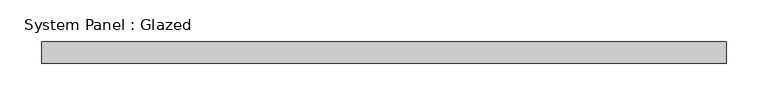
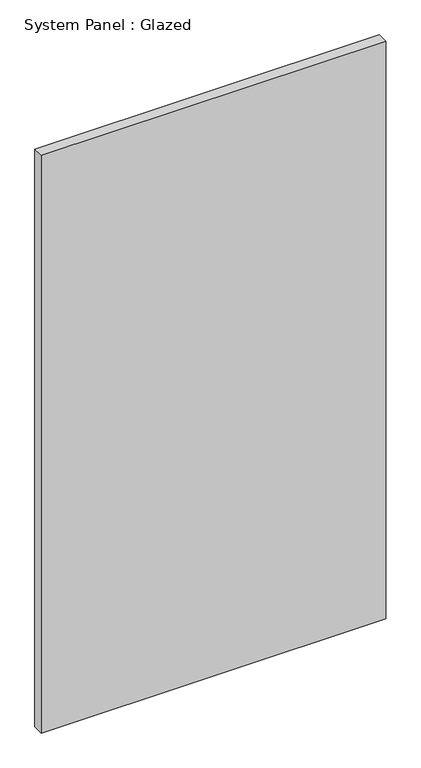
"""IFC4 building model written with IfcOpenShell, lengths in millimetres: plate geometry, System Panel : Glazed."""

from ifc_helpers import new_model, si_unit, origin, origin_with_axes, place, context, project, spatial, polyline, outline, extrude, source, transform, mapped, element, save


def system_panel_glazed_c67bbfce(model_context):
    return source(origin(), model_context, "Body", "SweptSolid", [
        extrude(outline(polyline([(409.575, 19.05), (-409.575, 19.05), (-409.575, 44.45), (409.575, 44.45), (409.575, 19.05)])), origin_with_axes(), (0.0, 0.0, 1.0), 1452.7129991),
    ])


if __name__ == "__main__":
    model = new_model("IFC4")
    model_context = context("Model", 3, world=origin())
    ifc_project = project(units=[si_unit("LENGTHUNIT", "METRE", prefix="MILLI")], contexts=[model_context])
    site = spatial("IfcSite", under=ifc_project)
    building = spatial("IfcBuilding", under=site)
    placement = place(None, origin())
    system_panel_glazed_shape = system_panel_glazed_c67bbfce(model_context)
    element("IfcPlate", 1, ObjectType="System Panel : Glazed", at=placement, inside=building, context=model_context, shape_type="MappedRepresentation", body=[
        mapped(system_panel_glazed_shape, transform((0.0, 0.0, 0.0), x_axis=(1.0, 0.0, 0.0), y_axis=(0.0, 1.0, 0.0), z_axis=(0.0, 0.0, 1.0))),
    ])
    save(model, "model.ifc")

# Revit data of these elements
# Type "System Panel : Glazed"
#   Construction Type Id = "GSP4R"
#   Analytic Construction = "1/8 in Pilkington single glazing"
#   Visual Light Transmittance = 0.9
#   Solar Heat Gain Coefficient = 0.86
#   Heat Transfer Coefficient (U) = 1.18115 BTU/(h·ft²·°F)
#   Define Thermal Properties by = 1
# Element 1 (IfcPlate, "System Panel : Glazed")
#   Materials on its faces: "Glass"
# Materials
#   "Glass": class "Glass", colour RGB 0 128 192, transparency 0.75, Description = "Soda Lime Glass", Cost = 0
